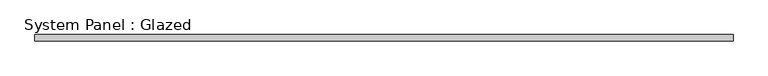
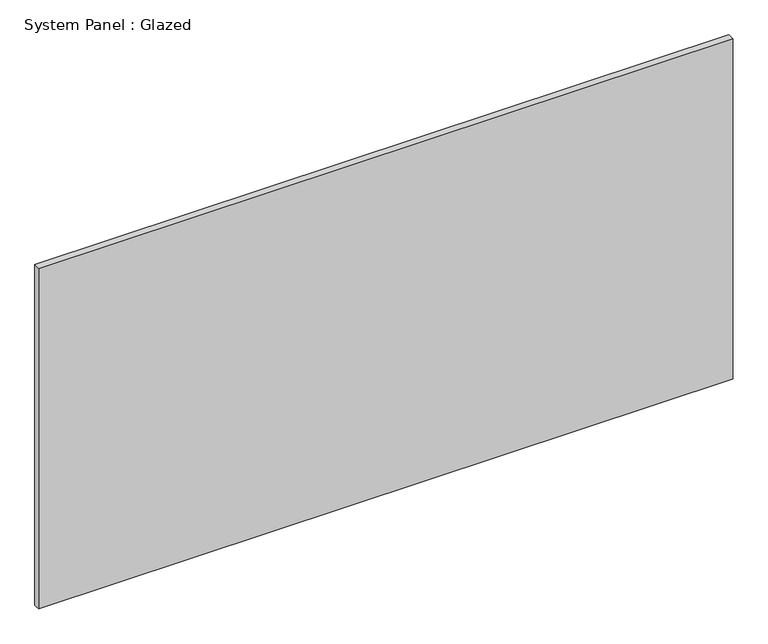
"""IFC4 building model written with IfcOpenShell, lengths in millimetres: plate geometry, System Panel : Glazed."""

from ifc_helpers import new_model, si_unit, origin, origin_with_axes, place, context, project, spatial, polyline, outline, extrude, source, transform, mapped, element, save


def system_panel_glazed_d483336f(model_context):
    return source(origin(), model_context, "Body", "SweptSolid", [
        extrude(outline(polyline([(1408.2170105, 19.05), (-1408.2170105, 19.05), (-1408.2170105, 44.45), (1408.2170105, 44.45), (1408.2170105, 19.05)])), origin_with_axes(), (0.0, 0.0, 1.0), 1460.5),
    ])


if __name__ == "__main__":
    model = new_model("IFC4")
    model_context = context("Model", 3, world=origin())
    ifc_project = project(units=[si_unit("LENGTHUNIT", "METRE", prefix="MILLI")], contexts=[model_context])
    site = spatial("IfcSite", under=ifc_project)
    building = spatial("IfcBuilding", under=site)
    placement = place(None, origin())
    system_panel_glazed_shape = system_panel_glazed_d483336f(model_context)
    element("IfcPlate", 1, ObjectType="System Panel : Glazed", at=placement, inside=building, context=model_context, shape_type="MappedRepresentation", body=[
        mapped(system_panel_glazed_shape, transform((0.0, 0.0, 0.0), x_axis=(1.0, 0.0, 0.0), y_axis=(0.0, 1.0, 0.0), z_axis=(0.0, 0.0, 1.0))),
    ])
    save(model, "model.ifc")

# Revit data of these elements
# Type "System Panel : Glazed"
#   Construction Type Id = "GSP4R"
#   Analytic Construction = "1/8 in Pilkington single glazing"
#   Visual Light Transmittance = 0.9
#   Solar Heat Gain Coefficient = 0.86
#   Heat Transfer Coefficient (U) = 1.18115 BTU/(h·ft²·°F)
#   Define Thermal Properties by = 1
# Element 1 (IfcPlate, "System Panel : Glazed")
#   Materials on its faces: "Glass"
# Materials
#   "Glass": class "Glass", colour RGB 0 128 192, transparency 0.75, Description = "Soda Lime Glass", Cost = 0
